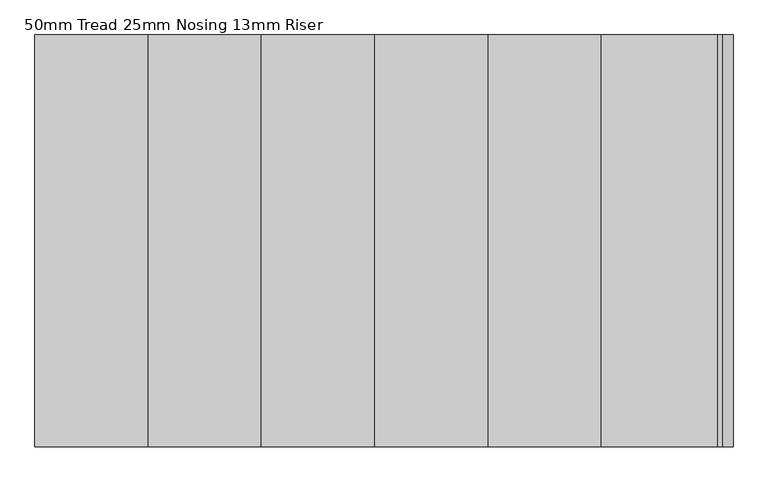
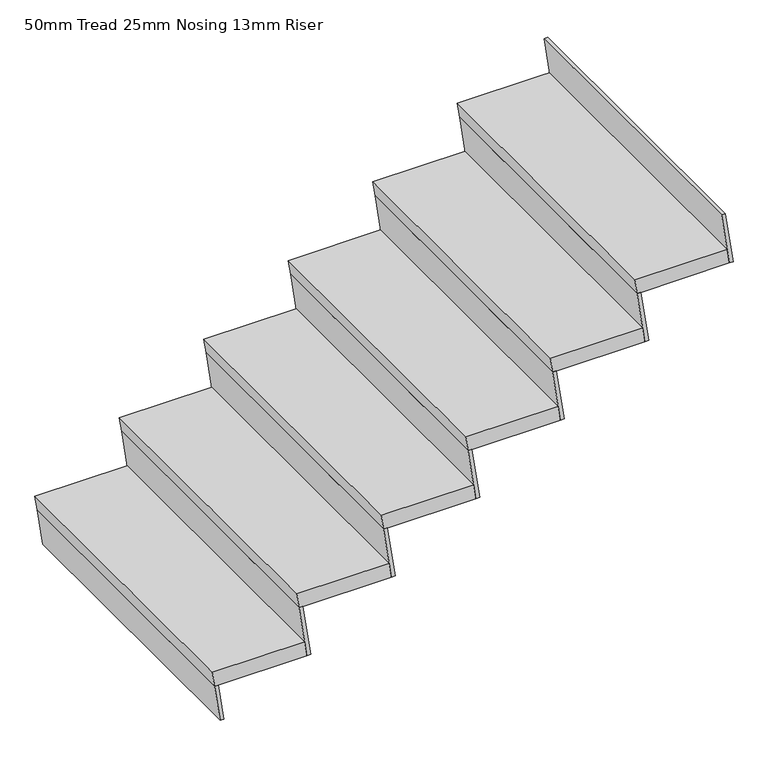
"""IFC4 building model written with IfcOpenShell, lengths in millimetres: stair flight geometry, 50mm Tread 25mm Nosing 13mm Riser."""

from ifc_helpers import new_model, si_unit, origin, place, context, project, spatial, faceted_brep, source, transform, mapped, element, save


def stair_flight_50mm_tread_25mm_nosing_13mm_riser_f0f518ff(model_context):
    return source(origin(), model_context, "Body", "Brep", [
        faceted_brep([(-8439.5726707, 1160.3053702, 173.9130435), (-8432.3851707, 1160.3053702, 123.9130435), (-8432.3851707, 2160.3311514, 123.9130435), (-8439.5726707, 2160.3311514, 173.9130435), (-8739.5726707, 2160.3311514, 173.9130435), (-8739.5726707, 1160.3053702, 173.9130435), (-8732.3851707, 1160.3053702, 123.9130435), (-8732.3851707, 2160.3311514, 123.9130435)], [[[0, 1, 2, 3]], [[3, 4, 5, 0]], [[2, 1, 6, 7]], [[4, 3, 2, 7]], [[0, 5, 6, 1]], [[5, 4, 7, 6]]]),
        faceted_brep([(-8732.3851707, 1160.3053702, 123.9130435), (-8714.5726707, 1160.3053702, 0.0), (-8701.9441807, 1160.3053702, 0.0), (-8719.7566807, 1160.3053702, 123.9130435), (-8732.3851707, 2160.3311514, 123.9130435), (-8719.7566807, 2160.3311514, 123.9130435), (-8701.9441807, 2160.3311514, 0.0), (-8714.5726707, 2160.3311514, 0.0)], [[[0, 1, 2, 3]], [[4, 5, 6, 7]], [[1, 0, 4, 7]], [[2, 1, 7, 6]], [[3, 2, 6, 5]], [[0, 3, 5, 4]]]),
        faceted_brep([(-8457.3851707, 1160.3053702, 297.826087), (-8432.3851707, 1160.3053702, 123.9130435), (-8419.7566807, 1160.3053702, 123.9130435), (-8444.7566807, 1160.3053702, 297.826087), (-8457.3851707, 2160.3311514, 297.826087), (-8444.7566807, 2160.3311514, 297.826087), (-8419.7566807, 2160.3311514, 123.9130435), (-8432.3851707, 2160.3311514, 123.9130435)], [[[0, 1, 2, 3]], [[4, 5, 6, 7]], [[1, 0, 4, 7]], [[2, 1, 7, 6]], [[3, 2, 6, 5]], [[0, 3, 5, 4]]]),
        faceted_brep([(-8164.5726707, 2160.3311514, 347.826087), (-8464.5726707, 2160.3311514, 347.826087), (-8464.5726707, 1160.3053702, 347.826087), (-8164.5726707, 1160.3053702, 347.826087), (-8157.3851707, 2160.3311514, 297.826087), (-8157.3851707, 1160.3053702, 297.826087), (-8457.3851707, 1160.3053702, 297.826087), (-8457.3851707, 2160.3311514, 297.826087)], [[[0, 1, 2, 3]], [[4, 5, 6, 7]], [[1, 0, 4, 7]], [[3, 2, 6, 5]], [[3, 5, 4, 0]], [[2, 1, 7, 6]]]),
        faceted_brep([(-8182.3851707, 1160.3053702, 471.7391304), (-8157.3851707, 1160.3053702, 297.826087), (-8144.7566807, 1160.3053702, 297.826087), (-8169.7566807, 1160.3053702, 471.7391304), (-8182.3851707, 2160.3311514, 471.7391304), (-8169.7566807, 2160.3311514, 471.7391304), (-8144.7566807, 2160.3311514, 297.826087), (-8157.3851707, 2160.3311514, 297.826087)], [[[0, 1, 2, 3]], [[4, 5, 6, 7]], [[1, 0, 4, 7]], [[2, 1, 7, 6]], [[3, 2, 6, 5]], [[0, 3, 5, 4]]]),
        faceted_brep([(-7889.5726707, 2160.3311514, 521.7391304), (-8189.5726707, 2160.3311514, 521.7391304), (-8189.5726707, 1160.3053702, 521.7391304), (-7889.5726707, 1160.3053702, 521.7391304), (-7882.3851707, 2160.3311514, 471.7391304), (-7882.3851707, 1160.3053702, 471.7391304), (-8182.3851707, 1160.3053702, 471.7391304), (-8182.3851707, 2160.3311514, 471.7391304)], [[[0, 1, 2, 3]], [[4, 5, 6, 7]], [[1, 0, 4, 7]], [[3, 2, 6, 5]], [[3, 5, 4, 0]], [[2, 1, 7, 6]]]),
        faceted_brep([(-7907.3851707, 1160.3053702, 645.6521739), (-7882.3851707, 1160.3053702, 471.7391304), (-7869.7566807, 1160.3053702, 471.7391304), (-7894.7566807, 1160.3053702, 645.6521739), (-7907.3851707, 2160.3311514, 645.6521739), (-7894.7566807, 2160.3311514, 645.6521739), (-7869.7566807, 2160.3311514, 471.7391304), (-7882.3851707, 2160.3311514, 471.7391304)], [[[0, 1, 2, 3]], [[4, 5, 6, 7]], [[1, 0, 4, 7]], [[2, 1, 7, 6]], [[3, 2, 6, 5]], [[0, 3, 5, 4]]]),
        faceted_brep([(-7614.5726707, 2160.3311514, 695.6521739), (-7914.5726707, 2160.3311514, 695.6521739), (-7914.5726707, 1160.3053702, 695.6521739), (-7614.5726707, 1160.3053702, 695.6521739), (-7607.3851707, 2160.3311514, 645.6521739), (-7607.3851707, 1160.3053702, 645.6521739), (-7907.3851707, 1160.3053702, 645.6521739), (-7907.3851707, 2160.3311514, 645.6521739)], [[[0, 1, 2, 3]], [[4, 5, 6, 7]], [[1, 0, 4, 7]], [[3, 2, 6, 5]], [[3, 5, 4, 0]], [[2, 1, 7, 6]]]),
        faceted_brep([(-7632.3851707, 1160.3053702, 819.5652174), (-7607.3851707, 1160.3053702, 645.6521739), (-7594.7566807, 1160.3053702, 645.6521739), (-7619.7566807, 1160.3053702, 819.5652174), (-7632.3851707, 2160.3311514, 819.5652174), (-7619.7566807, 2160.3311514, 819.5652174), (-7594.7566807, 2160.3311514, 645.6521739), (-7607.3851707, 2160.3311514, 645.6521739)], [[[0, 1, 2, 3]], [[4, 5, 6, 7]], [[1, 0, 4, 7]], [[2, 1, 7, 6]], [[3, 2, 6, 5]], [[0, 3, 5, 4]]]),
        faceted_brep([(-7339.5726707, 2160.3311514, 869.5652174), (-7639.5726707, 2160.3311514, 869.5652174), (-7639.5726707, 1160.3053702, 869.5652174), (-7339.5726707, 1160.3053702, 869.5652174), (-7332.3851707, 2160.3311514, 819.5652174), (-7332.3851707, 1160.3053702, 819.5652174), (-7632.3851707, 1160.3053702, 819.5652174), (-7632.3851707, 2160.3311514, 819.5652174)], [[[0, 1, 2, 3]], [[4, 5, 6, 7]], [[1, 0, 4, 7]], [[3, 2, 6, 5]], [[3, 5, 4, 0]], [[2, 1, 7, 6]]]),
        faceted_brep([(-7082.3851707, 1160.3053702, 1167.3913043), (-7057.3851707, 1160.3053702, 993.4782609), (-7044.7566807, 1160.3053702, 993.4782609), (-7069.7566807, 1160.3053702, 1167.3913043), (-7082.3851707, 2160.3311514, 1167.3913043), (-7069.7566807, 2160.3311514, 1167.3913043), (-7044.7566807, 2160.3311514, 993.4782609), (-7057.3851707, 2160.3311514, 993.4782609)], [[[0, 1, 2, 3]], [[4, 5, 6, 7]], [[1, 0, 4, 7]], [[2, 1, 7, 6]], [[3, 2, 6, 5]], [[0, 3, 5, 4]]]),
        faceted_brep([(-7357.3851707, 1160.3053702, 993.4782609), (-7332.3851707, 1160.3053702, 819.5652174), (-7319.7566807, 1160.3053702, 819.5652174), (-7344.7566807, 1160.3053702, 993.4782609), (-7357.3851707, 2160.3311514, 993.4782609), (-7344.7566807, 2160.3311514, 993.4782609), (-7319.7566807, 2160.3311514, 819.5652174), (-7332.3851707, 2160.3311514, 819.5652174)], [[[0, 1, 2, 3]], [[4, 5, 6, 7]], [[1, 0, 4, 7]], [[2, 1, 7, 6]], [[3, 2, 6, 5]], [[0, 3, 5, 4]]]),
        faceted_brep([(-7064.5726707, 2160.3311514, 1043.4782609), (-7089.5726707, 2160.3311514, 1043.4782609), (-7364.5726707, 2160.3311514, 1043.4782609), (-7364.5726707, 1160.3053702, 1043.4782609), (-7064.5726707, 1160.3053702, 1043.4782609), (-7057.3851707, 2160.3311514, 993.4782609), (-7057.3851707, 1160.3053702, 993.4782609), (-7357.3851707, 1160.3053702, 993.4782609), (-7357.3851707, 2160.3311514, 993.4782609), (-7089.5726707, 2160.3311514, 993.4782609)], [[[0, 1, 2, 3, 4]], [[5, 6, 7, 8, 9]], [[1, 0, 5, 9]], [[2, 1, 9, 8]], [[4, 3, 7, 6]], [[4, 6, 5, 0]], [[3, 2, 8, 7]]]),
    ])


if __name__ == "__main__":
    model = new_model("IFC4")
    model_context = context("Model", 3, world=origin())
    ifc_project = project(units=[si_unit("LENGTHUNIT", "METRE", prefix="MILLI")], contexts=[model_context])
    site = spatial("IfcSite", under=ifc_project)
    building = spatial("IfcBuilding", under=site)
    placement = place(None, origin())
    stair_flight_50mm_tread_25mm_nosing_13mm_riser_shape = stair_flight_50mm_tread_25mm_nosing_13mm_riser_f0f518ff(model_context)
    element("IfcStairFlight", 1, ObjectType="50mm Tread 25mm Nosing 13mm Riser", at=placement, inside=building, context=model_context, shape_type="MappedRepresentation", body=[
        mapped(stair_flight_50mm_tread_25mm_nosing_13mm_riser_shape, transform((0.0, 0.0, 0.0), x_axis=(1.0, 0.0, 0.0), y_axis=(0.0, 1.0, 0.0), z_axis=(0.0, 0.0, 1.0))),
    ])
    save(model, "model.ifc")
